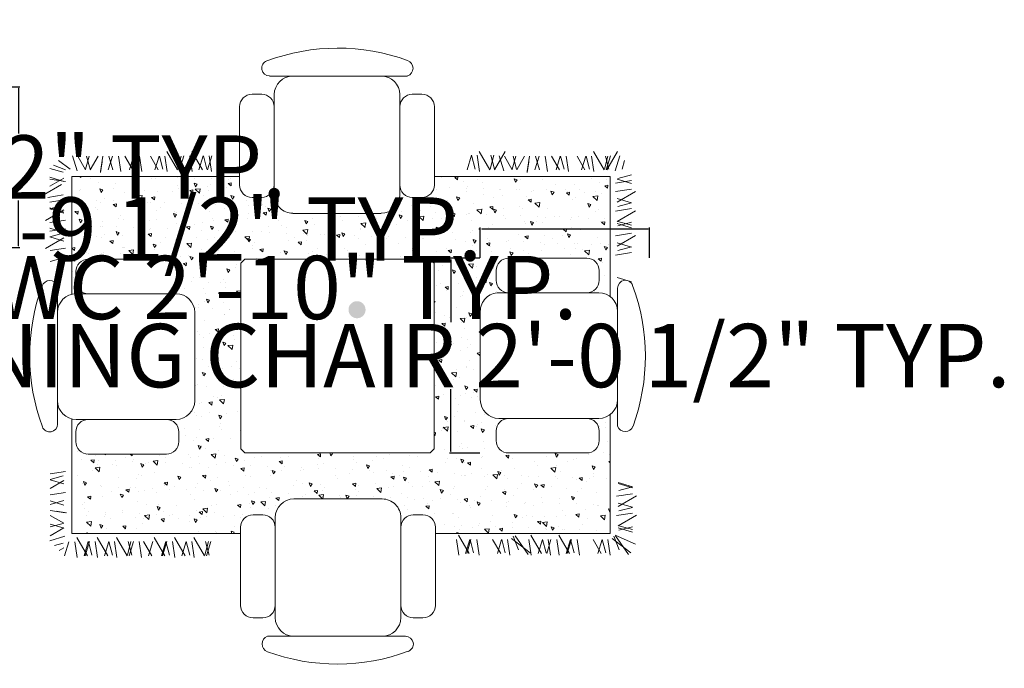
# Model space of a CAD drawing. Units: inches. Extents: x 638 to 1303, y 1 to 699.
# Tile 7 of 21: x 855 to 980, y 224 to 306. Entities that reach past the tile are written whole.
import ezdxf

# ---------------------------------------------------------------- set-up
doc = ezdxf.new("R2010")
doc.units = ezdxf.units.IN
doc.header["$MEASUREMENT"] = 0
for name, color, linetype, lineweight in [('A-ANNO-DIMS', 2, 'Continuous', 18), ('A-FURN-PATT', 8, 'Continuous', 13), ('A-FURN-RUGS', 8, 'Continuous', 13), ('Furniture', 7, 'Continuous', 15)]:
    doc.layers.add(name, color=color, linetype=linetype, lineweight=lineweight)
doc.styles.get("Standard").update_dxf_attribs({"font": 'arial.ttf'})
doc.dimstyles.get("Standard").update_dxf_attribs({"dimtxt": 8, "dimasz": 0.18, "dimexe": 0.18, "dimexo": 0.0625, "dimgap": 0.09, "dimtad": 0, "dimtih": 1, "dimtoh": 1, "dimdec": 4, "dimzin": 0, "dimdsep": 46, "dimlunit": 3, "dimtxsty": 'Standard', "dimcen": 0.09, "dimadec": 0, "dimazin": 0, "dimtfac": 1, "dimtdec": 4, "dimtofl": 0, "dimtmove": 0, "dimatfit": 3, "dimfxl": 1, "dimtolj": 1, "dimtzin": 0, "dimarcsym": 0})

# ---------------------------------------------------------------- blocks, each defined once
blk = doc.blocks.new('CHAIR-UPHOLSTERED')
for p, q in [((7.4, 24.61, 7.15), (17.29, 24.61, 7.15)), ((5.82, 21.82, 7.15), (5.82, 23.04, 7.15)), ((18.86, 23.04, 7.15), (18.86, 21.82, 7.15)), ((3.52, 21.23, 7.15), (3.52, 4.36, 7.15)), ((5.87, 20.25, 7.15), (18.51, 20.25, 7.15)), ((17.29, 20.25, 7.15), (7.4, 20.25, 7.15)), ((3.52, 6.72, 7.15), (3.52, 17.89, 7.15)), ((20.87, 17.89, 7.15), (20.87, 6.72, 7.15)), ((3.52, 4.36, 7.15), (3.52, 3.77, 7.15)), ((18.51, 4.36, 7.15), (5.87, 4.36, 7.15)), ((7.4, 4.36, 7.15), (17.29, 4.36, 7.15)), ((5.82, 1.57, 7.15), (5.82, 2.79, 7.15)), ((18.86, 2.79, 7.15), (18.86, 1.57, 7.15)), ((17.29, 0, 7.15), (7.4, 0, 7.15))]:
    blk.add_line(p, q)
for centre, radius, start, end in [((7.4, 23.04, 7.15), 1.57, 90, 180), ((17.29, 23.04, 7.15), 1.57, 0, 90), ((25.77, 12.4, 7.15), 25.77, 159.9544, 200.3611), ((2.54, 20.87, 7.15), 1.04, 20.0456, 159.9544), ((7.4, 21.82, 7.15), 1.57, 180, 270), ((17.29, 21.82, 7.15), 1.57, 270, 0), ((5.87, 17.89, 7.15), 2.35, 90, 180), ((18.51, 17.89, 7.15), 2.35, 0, 90), ((5.87, 6.72, 7.15), 2.35, 180, 270), ((18.51, 6.72, 7.15), 2.35, 270, 0), ((2.53, 3.77, 7.15), 0.986, 200.3611, 0), ((7.4, 2.79, 7.15), 1.57, 90, 180), ((17.29, 2.79, 7.15), 1.57, 0, 90), ((7.4, 1.57, 7.15), 1.57, 180, 270), ((17.29, 1.57, 7.15), 1.57, 270, 0)]:
    blk.add_arc(centre, radius, start, end)
blk = doc.blocks.new('*D30')
at = {"layer": 'A-ANNO-DIMS', "color": 0, "lineweight": -2, "transparency": 16777216}
for p, q in [((913.6, 276.19), (909.79, 276.19)), ((909.97, 276.01), (909.97, 268.11)), ((909.97, 251.76), (909.97, 259.66)), ((913.6, 251.58), (909.79, 251.58))]:
    blk.add_line(p, q, dxfattribs=at)
at = {"layer": 'A-ANNO-DIMS', "color": 0, "transparency": 16777216}
for points in [[(909.94, 276.01), (910, 276.01), (909.97, 276.19)], [(909.94, 251.76), (910, 251.76), (909.97, 251.58)]]:
    blk.add_solid(points, dxfattribs=at)
at = {"layer": 'Defpoints', "color": 0, "transparency": 16777216}
for p in [(913.67, 276.19), (909.97, 251.58), (913.67, 251.58)]:
    blk.add_point(p, dxfattribs=at)
at = {"layer": 'A-ANNO-DIMS', "color": 0, "transparency": 16777216, "insert": (909.97, 263.89), "char_height": 8, "attachment_point": 5}
blk.add_mtext('\\A1;DINING CHAIR 2\'-0 1/2" TYP.', dxfattribs=at)
blk = doc.blocks.new('*D31')
at = {"layer": 'A-ANNO-DIMS', "color": 0, "lineweight": -2, "transparency": 16777216}
for p, q in [((913.67, 276.25), (913.67, 280.06)), ((935.07, 276.25), (935.07, 280.06)), ((913.67, 279.88), (913.49, 279.88)), ((934.89, 279.88), (913.85, 279.88))]:
    blk.add_line(p, q, dxfattribs=at)
at = {"layer": 'A-ANNO-DIMS', "color": 0, "transparency": 16777216}
for points in [[(913.85, 279.91), (913.85, 279.85), (913.67, 279.88)], [(934.89, 279.91), (934.89, 279.85), (935.07, 279.88)]]:
    blk.add_solid(points, dxfattribs=at)
at = {"layer": 'Defpoints', "color": 0, "transparency": 16777216}
for p in [(913.67, 279.88), (913.67, 276.19), (935.07, 276.19)]:
    blk.add_point(p, dxfattribs=at)
at = {"layer": 'A-ANNO-DIMS', "color": 0, "transparency": 16777216, "insert": (880.07, 279.88), "char_height": 8, "attachment_point": 5}
blk.add_mtext('\\A1;1\'-9 1/2" TYP.', dxfattribs=at)
blk = doc.blocks.new('*D32')
at = {"layer": 'A-ANNO-DIMS', "color": 0, "lineweight": -2, "transparency": 16777216}
for p, q in [((816.4, 277.5), (816.4, 272.31)), ((850.23, 277.5), (850.23, 272.31)), ((816.58, 272.49), (850.05, 272.49)), ((850.23, 272.49), (850.41, 272.49))]:
    blk.add_line(p, q, dxfattribs=at)
at = {"layer": 'A-ANNO-DIMS', "color": 0, "transparency": 16777216}
for points in [[(816.58, 272.52), (816.58, 272.46), (816.4, 272.49)], [(850.05, 272.52), (850.05, 272.46), (850.23, 272.49)]]:
    blk.add_solid(points, dxfattribs=at)
at = {"layer": 'Defpoints', "color": 0, "transparency": 16777216}
for p in [(816.4, 277.56), (850.23, 277.56), (850.23, 272.49)]:
    blk.add_point(p, dxfattribs=at)
at = {"layer": 'A-ANNO-DIMS', "color": 0, "transparency": 16777216, "insert": (889.02, 272.49), "char_height": 8, "attachment_point": 5}
blk.add_mtext('\\A1;WC 2\'-10" TYP.', dxfattribs=at)
blk = doc.blocks.new('*D33')
at = {"layer": 'A-ANNO-DIMS', "color": 0, "lineweight": -2, "transparency": 16777216}
for p, q in [((850.3, 297.86), (855.49, 297.86)), ((855.31, 297.68), (855.31, 291.94)), ((855.31, 277.74), (855.31, 283.49)), ((850.3, 277.56), (855.49, 277.56))]:
    blk.add_line(p, q, dxfattribs=at)
at = {"layer": 'A-ANNO-DIMS', "color": 0, "transparency": 16777216}
for points in [[(855.28, 297.68), (855.34, 297.68), (855.31, 297.86)], [(855.28, 277.74), (855.34, 277.74), (855.31, 277.56)]]:
    blk.add_solid(points, dxfattribs=at)
at = {"layer": 'Defpoints', "color": 0, "transparency": 16777216}
for p in [(850.23, 297.86), (855.31, 297.86), (850.23, 277.56)]:
    blk.add_point(p, dxfattribs=at)
at = {"layer": 'A-ANNO-DIMS', "color": 0, "transparency": 16777216, "insert": (855.31, 287.71), "char_height": 8, "attachment_point": 5}
blk.add_mtext('\\A1;1\'-8 1/2" TYP.', dxfattribs=at)

msp = doc.modelspace()

# ---------------------------------------------------------------- hatches: boundary and pattern name
at = {"layer": 'A-FURN-PATT'}
h = msp.add_hatch(dxfattribs=at)
h.set_pattern_fill('AR-CONC', color=256, scale=0.643499, angle=90, style=0)
h.set_pattern_definition([(140, (0, 0), (0.403809, 4.61556), [0.482624, -5.308864]), (85, (0, 0), (-4.840347, -0.892863), [0.3861, -4.247092]), (190.45144, (0.0337, 0.3846), (-4.436537, 3.722697), [0.410167, -4.51184]), (136.1842, (-1.287, 1e-16), (1.065114, 6.867684), [0.723936, -7.963297]), (186.6356, (-1.198, 0.572), (-6.26844, 6.014538), [0.61525, -6.767765]), (81.1842, (-1.287, 1e-16), (-6.26844, 6.01454), [0.57915, -6.370637]), (111, (-0.9652, 0.6435), (2.590847, 3.841089), [0.482624, -5.308864]), (56, (-0.9652, 0.6435), (-4.666331, 1.56573), [0.3861, -4.247092]), (161.45144, (-0.7493, 0.9636), (-2.075484, 5.40682), [0.410167, -4.51184]), (127.5, (0, 0), (-2.1421677, 0.0782485), [0, -4.1956116, 0, -4.3114414, 0, -4.263179]), (97.5, (0, 0), (-2.5380343, 1.692849), [0, -2.458165, 0, -4.099087, 0, -1.624834]), (57.5, (-1e-16, -1.435), (0.1451403, 3.4351405), [0, -1.608747, 0, -5.01929, 0, -6.660212]), (47.5, (-1e-16, -2.0785), (-0.644174, 3.7527955), [0, -2.091371, 0, -3.333323, 0, -4.729716])])
h.paths.add_polyline_path([(883.26022, 286.50863), (862.04846, 286.50863), (862.04846, 271.63405), (862.11053, 271.64895), (862.23163, 271.67139), (862.35374, 271.68747), (862.47652, 271.69713), (862.59965, 271.70036), (864.1212, 271.70036), (864.03898, 271.70251), (863.95698, 271.70896), (863.87543, 271.7197), (863.79456, 271.73469), (863.71458, 271.75389), (863.63572, 271.77725), (863.55818, 271.80471), (863.48219, 271.83618), (863.40795, 271.87159), (863.33567, 271.91084), (863.26554, 271.95382), (863.19775, 272.00041), (863.1325, 272.05048), (863.06995, 272.10389), (863.01029, 272.16051), (862.95367, 272.22018), (862.90025, 272.28272), (862.85018, 272.34798), (862.80359, 272.41576), (862.76062, 272.48589), (862.72137, 272.55818), (862.68596, 272.63241), (862.65448, 272.70841), (862.62703, 272.78594), (862.60367, 272.8648), (862.58447, 272.94478), (862.56948, 273.02566), (862.55874, 273.1072), (862.55229, 273.1892), (862.55013, 273.27143), (862.55013, 274.49251), (862.55229, 274.57473), (862.55874, 274.65673), (862.56948, 274.73828), (862.58447, 274.81915), (862.60367, 274.89913), (862.62703, 274.978), (862.65448, 275.05553), (862.68596, 275.13152), (862.72137, 275.20576), (862.76062, 275.27804), (862.80359, 275.34817), (862.85018, 275.41596), (862.90025, 275.48121), (862.95367, 275.54376), (863.01029, 275.60342), (863.06995, 275.66004), (863.1325, 275.71346), (863.19775, 275.76353), (863.26554, 275.81012), (863.33567, 275.85309), (863.40795, 275.89234), (863.48219, 275.92775), (863.55818, 275.95923), (863.63572, 275.98668), (863.71458, 276.01004), (863.79456, 276.02925), (863.87543, 276.04424), (863.95698, 276.05497), (864.03898, 276.06142), (864.1212, 276.06358), (874.01311, 276.06358), (874.09533, 276.06142), (874.17733, 276.05497), (874.25888, 276.04424), (874.33975, 276.02925), (874.41973, 276.01004), (874.4986, 275.98668), (874.57613, 275.95923), (874.65212, 275.92775), (874.72636, 275.89234), (874.79864, 275.85309), (874.86878, 275.81012), (874.93656, 275.76353), (875.00182, 275.71346), (875.06436, 275.66004), (875.12402, 275.60342), (875.18064, 275.54376), (875.23406, 275.48121), (875.28413, 275.41596), (875.33072, 275.34817), (875.3737, 275.27804), (875.41294, 275.20576), (875.44835, 275.13152), (875.47983, 275.05553), (875.50729, 274.978), (875.53065, 274.89913), (875.54985, 274.81915), (875.56484, 274.73828), (875.57557, 274.65673), (875.58203, 274.57473), (875.58418, 274.49251), (875.58418, 273.27143), (875.58203, 273.1892), (875.57557, 273.1072), (875.56484, 273.02566), (875.54985, 272.94478), (875.53065, 272.8648), (875.50729, 272.78594), (875.47983, 272.70841), (875.44835, 272.63241), (875.41294, 272.55818), (875.3737, 272.48589), (875.33072, 272.41576), (875.28413, 272.34798), (875.23406, 272.28272), (875.18064, 272.22018), (875.12402, 272.16051), (875.06436, 272.10389), (875.00182, 272.05048), (874.93656, 272.00041), (874.86878, 271.95382), (874.79864, 271.91084), (874.72636, 271.87159), (874.65212, 271.83618), (874.57613, 271.80471), (874.4986, 271.77725), (874.41973, 271.75389), (874.33975, 271.73469), (874.25888, 271.7197), (874.17733, 271.70896), (874.09533, 271.70251), (874.01311, 271.70036), (875.24067, 271.70036), (875.36379, 271.69713), (875.48657, 271.68747), (875.60868, 271.67139), (875.72978, 271.64895), (875.84954, 271.6202), (875.96763, 271.58522), (876.08373, 271.5441), (876.19752, 271.49697), (876.30869, 271.44395), (876.41693, 271.38518), (876.52194, 271.32083), (876.62344, 271.25107), (876.72115, 271.17609), (876.81481, 271.0961), (876.90415, 271.01132), (876.98893, 270.92198), (877.06892, 270.82833), (877.14389, 270.73061), (877.21365, 270.62911), (877.27801, 270.5241), (877.33678, 270.41586), (877.3898, 270.30469), (877.43693, 270.19091), (877.47804, 270.07481), (877.51303, 269.95672), (877.54178, 269.83696), (877.56422, 269.71585), (877.5803, 269.59374), (877.58996, 269.47096), (877.59319, 269.34784), (877.59319, 258.1688), (877.58996, 258.04567), (877.5803, 257.92289), (877.56422, 257.80078), (877.54178, 257.67968), (877.51303, 257.55992), (877.47804, 257.44183), (877.43693, 257.32573), (877.3898, 257.21194), (877.33678, 257.10077), (877.27801, 256.99254), (877.21365, 256.88752), (877.14389, 256.78602), (877.06892, 256.68831), (876.98893, 256.59465), (876.90415, 256.50531), (876.81481, 256.42053), (876.72115, 256.34054), (876.62344, 256.26557), (876.52194, 256.19581), (876.41693, 256.13145), (876.30869, 256.07269), (876.19752, 256.01966), (876.08373, 255.97253), (875.96763, 255.93142), (875.84954, 255.89644), (875.72978, 255.86768), (875.60868, 255.84524), (875.48657, 255.82916), (875.36379, 255.8195), (875.24067, 255.81628), (874.01311, 255.81628), (874.09533, 255.81412), (874.17733, 255.80767), (874.25888, 255.79693), (874.33975, 255.78194), (874.41973, 255.76274), (874.4986, 255.73938), (874.57613, 255.71193), (874.65212, 255.68045), (874.72636, 255.64504), (874.79864, 255.60579), (874.86878, 255.56282), (874.93656, 255.51623), (875.00182, 255.46616), (875.06436, 255.41274), (875.12402, 255.35612), (875.18064, 255.29646), (875.23406, 255.23391), (875.28413, 255.16866), (875.33072, 255.10087), (875.3737, 255.03074), (875.41294, 254.95846), (875.44835, 254.88422), (875.47983, 254.80823), (875.50729, 254.73069), (875.53065, 254.65183), (875.54985, 254.57185), (875.56484, 254.49098), (875.57557, 254.40943), (875.58203, 254.32743), (875.58418, 254.24521), (875.58418, 253.02412), (875.58203, 252.9419), (875.57557, 252.8599), (875.56484, 252.77836), (875.54985, 252.69748), (875.53065, 252.6175), (875.50729, 252.53864), (875.47983, 252.4611), (875.44835, 252.38511), (875.41294, 252.31087), (875.3737, 252.23859), (875.33072, 252.16846), (875.28413, 252.10067), (875.23406, 252.03542), (875.18064, 251.97287), (875.12402, 251.91321), (875.06436, 251.85659), (875.00182, 251.80318), (874.93656, 251.7531), (874.86878, 251.70652), (874.79864, 251.66354), (874.72636, 251.62429), (874.65212, 251.58888), (874.57613, 251.55741), (874.4986, 251.52995), (874.41973, 251.50659), (874.33975, 251.48739), (874.25888, 251.4724), (874.17733, 251.46166), (874.09533, 251.45521), (874.01311, 251.45306), (864.1212, 251.45306), (864.03898, 251.45521), (863.95698, 251.46166), (863.87543, 251.4724), (863.79456, 251.48739), (863.71458, 251.50659), (863.63572, 251.52995), (863.55818, 251.55741), (863.48219, 251.58888), (863.40795, 251.62429), (863.33567, 251.66354), (863.26554, 251.70652), (863.19775, 251.7531), (863.1325, 251.80318), (863.06995, 251.85659), (863.01029, 251.91321), (862.95367, 251.97287), (862.90025, 252.03542), (862.85018, 252.10067), (862.80359, 252.16846), (862.76062, 252.23859), (862.72137, 252.31087), (862.68596, 252.38511), (862.65448, 252.4611), (862.62703, 252.53864), (862.60367, 252.6175), (862.58447, 252.69748), (862.56948, 252.77836), (862.55874, 252.8599), (862.55229, 252.9419), (862.55013, 253.02412), (862.55013, 254.24521), (862.55229, 254.32743), (862.55874, 254.40943), (862.56948, 254.49098), (862.58447, 254.57185), (862.60367, 254.65183), (862.62703, 254.73069), (862.65448, 254.80823), (862.68596, 254.88422), (862.72137, 254.95846), (862.76062, 255.03074), (862.80359, 255.10087), (862.85018, 255.16866), (862.90025, 255.23391), (862.95367, 255.29646), (863.01029, 255.35612), (863.06995, 255.41274), (863.1325, 255.46616), (863.19775, 255.51623), (863.26554, 255.56282), (863.33567, 255.60579), (863.40795, 255.64504), (863.48219, 255.68045), (863.55818, 255.71193), (863.63572, 255.73938), (863.71458, 255.76274), (863.79456, 255.78194), (863.87543, 255.79693), (863.95698, 255.80767), (864.03898, 255.81412), (864.1212, 255.81628), (862.59965, 255.81628), (862.47652, 255.8195), (862.35374, 255.82916), (862.23163, 255.84524), (862.11053, 255.86768), (862.04846, 255.88259), (862.04846, 241.41532), (883.3886, 241.41532), (883.3886, 242.20595), (883.39075, 242.28817), (883.39721, 242.37017), (883.40794, 242.45172), (883.42293, 242.53259), (883.44213, 242.61257), (883.4655, 242.69144), (883.49295, 242.76897), (883.52443, 242.84496), (883.55984, 242.9192), (883.59909, 242.99149), (883.64206, 243.06162), (883.68865, 243.1294), (883.73872, 243.19466), (883.79214, 243.2572), (883.84876, 243.31686), (883.90842, 243.37348), (883.97096, 243.4269), (884.03622, 243.47697), (884.104, 243.52356), (884.17414, 243.56654), (884.24642, 243.60578), (884.32066, 243.64119), (884.39665, 243.67267), (884.47418, 243.70013), (884.55305, 243.72349), (884.63303, 243.74269), (884.7139, 243.75768), (884.79545, 243.76841), (884.87745, 243.77487), (884.95967, 243.77702), (886.18075, 243.77702), (886.26298, 243.77487), (886.34498, 243.76841), (886.42652, 243.75768), (886.5074, 243.74269), (886.58738, 243.72349), (886.66624, 243.70013), (886.74377, 243.67267), (886.81976, 243.64119), (886.894, 243.60578), (886.96629, 243.56654), (887.03642, 243.52356), (887.1042, 243.47697), (887.16946, 243.4269), (887.232, 243.37348), (887.29167, 243.31686), (887.34828, 243.2572), (887.4017, 243.19466), (887.45177, 243.1294), (887.49836, 243.06162), (887.54134, 242.99149), (887.58059, 242.9192), (887.616, 242.84496), (887.64747, 242.76897), (887.67493, 242.69144), (887.69829, 242.61257), (887.71749, 242.53259), (887.73248, 242.45172), (887.74322, 242.37017), (887.74967, 242.28817), (887.75182, 242.20595), (887.75182, 243.43351), (887.75505, 243.55663), (887.76471, 243.67941), (887.78079, 243.80152), (887.80323, 243.92262), (887.83198, 244.04238), (887.86696, 244.16048), (887.90808, 244.27657), (887.95521, 244.39036), (888.00823, 244.50153), (888.067, 244.60977), (888.13135, 244.71478), (888.20111, 244.81628), (888.27609, 244.914), (888.35608, 245.00765), (888.44086, 245.09699), (888.5302, 245.18177), (888.62385, 245.26176), (888.72156, 245.33674), (888.82307, 245.4065), (888.92808, 245.47085), (889.03632, 245.52962), (889.14749, 245.58264), (889.26127, 245.62977), (889.37737, 245.67089), (889.49546, 245.70587), (889.61522, 245.73462), (889.73633, 245.75706), (889.85844, 245.77314), (889.98122, 245.7828), (890.10434, 245.78603), (901.28338, 245.78603), (901.40651, 245.7828), (901.52929, 245.77314), (901.6514, 245.75706), (901.7725, 245.73462), (901.89226, 245.70587), (902.01035, 245.67089), (902.12645, 245.62977), (902.24024, 245.58264), (902.35141, 245.52962), (902.45964, 245.47085), (902.56466, 245.4065), (902.66616, 245.33674), (902.76387, 245.26176), (902.85753, 245.18177), (902.94687, 245.09699), (903.03165, 245.00765), (903.11163, 244.914), (903.18661, 244.81628), (903.25637, 244.71478), (903.32073, 244.60977), (903.37949, 244.50153), (903.43252, 244.39036), (903.47965, 244.27657), (903.52076, 244.16048), (903.55574, 244.04238), (903.5845, 243.92262), (903.60694, 243.80152), (903.62302, 243.67941), (903.63268, 243.55663), (903.6359, 243.43351), (903.6359, 242.20595), (903.63806, 242.28817), (903.64451, 242.37017), (903.65525, 242.45172), (903.67023, 242.53259), (903.68944, 242.61257), (903.7128, 242.69144), (903.74025, 242.76897), (903.77173, 242.84496), (903.80714, 242.9192), (903.84639, 242.99149), (903.88936, 243.06162), (903.93595, 243.1294), (903.98602, 243.19466), (904.03944, 243.2572), (904.09606, 243.31686), (904.15572, 243.37348), (904.21827, 243.4269), (904.28352, 243.47697), (904.35131, 243.52356), (904.42144, 243.56654), (904.49372, 243.60578), (904.56796, 243.64119), (904.64395, 243.67267), (904.72148, 243.70013), (904.80035, 243.72349), (904.88033, 243.74269), (904.9612, 243.75768), (905.04275, 243.76841), (905.12475, 243.77487), (905.20697, 243.77702), (906.42806, 243.77702), (906.51028, 243.77487), (906.59228, 243.76841), (906.67382, 243.75768), (906.7547, 243.74269), (906.83468, 243.72349), (906.91354, 243.70013), (906.99108, 243.67267), (907.06707, 243.64119), (907.14131, 243.60578), (907.21359, 243.56654), (907.28372, 243.52356), (907.35151, 243.47697), (907.41676, 243.4269), (907.4793, 243.37348), (907.53897, 243.31686), (907.59559, 243.2572), (907.649, 243.19466), (907.69908, 243.1294), (907.74566, 243.06162), (907.78864, 242.99149), (907.82789, 242.9192), (907.8633, 242.84496), (907.89477, 242.76897), (907.92223, 242.69144), (907.94559, 242.61257), (907.96479, 242.53259), (907.97978, 242.45172), (907.99052, 242.37017), (907.99697, 242.28817), (907.99912, 242.20595), (907.99912, 241.41532), (930.08632, 241.41532), (930.08632, 256.4276), (930.04247, 256.39395), (929.94097, 256.32419), (929.83595, 256.25984), (929.72771, 256.20107), (929.61655, 256.14805), (929.50276, 256.10092), (929.38666, 256.0598), (929.26857, 256.02482), (929.14881, 255.99607), (929.02771, 255.97363), (928.9056, 255.95755), (928.78281, 255.94789), (928.65969, 255.94466), (927.13814, 255.94466), (927.22036, 255.94251), (927.30236, 255.93606), (927.38391, 255.92532), (927.46478, 255.91033), (927.54476, 255.89113), (927.62362, 255.86777), (927.70116, 255.84031), (927.77715, 255.80884), (927.85139, 255.77343), (927.92367, 255.73418), (927.9938, 255.6912), (928.06159, 255.64462), (928.12684, 255.59454), (928.18939, 255.54113), (928.24905, 255.48451), (928.30567, 255.42484), (928.35909, 255.3623), (928.40916, 255.29705), (928.45575, 255.22926), (928.49872, 255.15913), (928.53797, 255.08684), (928.57338, 255.01261), (928.60485, 254.93662), (928.63231, 254.85908), (928.65567, 254.78022), (928.67487, 254.70024), (928.68986, 254.61936), (928.7006, 254.53782), (928.70705, 254.45582), (928.7092, 254.37359), (928.7092, 253.15251), (928.70705, 253.07029), (928.7006, 252.98829), (928.68986, 252.90674), (928.67487, 252.82587), (928.65567, 252.74589), (928.63231, 252.66702), (928.60485, 252.58949), (928.57338, 252.5135), (928.53797, 252.43926), (928.49872, 252.36698), (928.45575, 252.29685), (928.40916, 252.22906), (928.35909, 252.16381), (928.30567, 252.10126), (928.24905, 252.0416), (928.18939, 251.98498), (928.12684, 251.93156), (928.06159, 251.88149), (927.9938, 251.8349), (927.92367, 251.79193), (927.85139, 251.75268), (927.77715, 251.71727), (927.70116, 251.68579), (927.62362, 251.65834), (927.54476, 251.63498), (927.46478, 251.61577), (927.38391, 251.60079), (927.30236, 251.59005), (927.22036, 251.5836), (927.13814, 251.58144), (917.24623, 251.58144), (917.164, 251.5836), (917.08201, 251.59005), (917.00046, 251.60079), (916.91958, 251.61577), (916.83961, 251.63498), (916.76074, 251.65834), (916.68321, 251.68579), (916.60722, 251.71727), (916.53298, 251.75268), (916.46069, 251.79193), (916.39056, 251.8349), (916.32278, 251.88149), (916.25752, 251.93156), (916.19498, 251.98498), (916.13532, 252.0416), (916.0787, 252.10126), (916.02528, 252.16381), (915.97521, 252.22906), (915.92862, 252.29685), (915.88564, 252.36698), (915.8464, 252.43926), (915.81099, 252.5135), (915.77951, 252.58949), (915.75205, 252.66702), (915.72869, 252.74589), (915.70949, 252.82587), (915.6945, 252.90674), (915.68377, 252.98829), (915.67731, 253.07029), (915.67516, 253.15251), (915.67516, 254.37359), (915.67731, 254.45582), (915.68377, 254.53782), (915.6945, 254.61936), (915.70949, 254.70024), (915.72869, 254.78022), (915.75205, 254.85908), (915.77951, 254.93662), (915.81099, 255.01261), (915.8464, 255.08684), (915.88564, 255.15913), (915.92862, 255.22926), (915.97521, 255.29705), (916.02528, 255.3623), (916.0787, 255.42484), (916.13532, 255.48451), (916.19498, 255.54113), (916.25752, 255.59454), (916.32278, 255.64462), (916.39056, 255.6912), (916.46069, 255.73418), (916.53298, 255.77343), (916.60722, 255.80884), (916.68321, 255.84031), (916.76074, 255.86777), (916.83961, 255.89113), (916.91958, 255.91033), (917.00046, 255.92532), (917.08201, 255.93606), (917.164, 255.94251), (917.24623, 255.94466), (916.01867, 255.94466), (915.89555, 255.94789), (915.77277, 255.95755), (915.65066, 255.97363), (915.52956, 255.99607), (915.4098, 256.02482), (915.2917, 256.0598), (915.1756, 256.10092), (915.06182, 256.14805), (914.95065, 256.20107), (914.84241, 256.25984), (914.7374, 256.32419), (914.6359, 256.39395), (914.53818, 256.46893), (914.44453, 256.54892), (914.35519, 256.6337), (914.27041, 256.72304), (914.19042, 256.81669), (914.11544, 256.91441), (914.04568, 257.01591), (913.98133, 257.12092), (913.92256, 257.22916), (913.86954, 257.34033), (913.82241, 257.45411), (913.78129, 257.57021), (913.74631, 257.6883), (913.71756, 257.80807), (913.69512, 257.92917), (913.67904, 258.05128), (913.66938, 258.17406), (913.66615, 258.29718), (913.66615, 269.47623), (913.66938, 269.59935), (913.67904, 269.72213), (913.69512, 269.84424), (913.71756, 269.96534), (913.74631, 270.0851), (913.78129, 270.20319), (913.82241, 270.31929), (913.86954, 270.43308), (913.92256, 270.54425), (913.98133, 270.65248), (914.04568, 270.7575), (914.11544, 270.859), (914.19042, 270.95671), (914.27041, 271.05037), (914.35519, 271.13971), (914.44453, 271.22449), (914.53818, 271.30448), (914.6359, 271.37945), (914.7374, 271.44921), (914.84241, 271.51357), (914.95065, 271.57234), (915.06182, 271.62536), (915.1756, 271.67249), (915.2917, 271.7136), (915.4098, 271.74858), (915.52956, 271.77734), (915.65066, 271.79978), (915.77277, 271.81586), (915.89555, 271.82552), (916.01867, 271.82874), (917.24623, 271.82874), (917.164, 271.8309), (917.08201, 271.83735), (917.00046, 271.84809), (916.91958, 271.86308), (916.83961, 271.88228), (916.76074, 271.90564), (916.68321, 271.93309), (916.60722, 271.96457), (916.53298, 271.99998), (916.46069, 272.03923), (916.39056, 272.0822), (916.32278, 272.12879), (916.25752, 272.17886), (916.19498, 272.23228), (916.13532, 272.2889), (916.0787, 272.34856), (916.02528, 272.41111), (915.97521, 272.47636), (915.92862, 272.54415), (915.88564, 272.61428), (915.8464, 272.68656), (915.81099, 272.7608), (915.77951, 272.83679), (915.75205, 272.91433), (915.72869, 272.99319), (915.70949, 273.07317), (915.6945, 273.15404), (915.68377, 273.23559), (915.67731, 273.31759), (915.67516, 273.39981), (915.67516, 274.6209), (915.67731, 274.70312), (915.68377, 274.78512), (915.6945, 274.86667), (915.70949, 274.94754), (915.72869, 275.02752), (915.75205, 275.10638), (915.77951, 275.18392), (915.81099, 275.25991), (915.8464, 275.33415), (915.88564, 275.40643), (915.92862, 275.47656), (915.97521, 275.54435), (916.02528, 275.6096), (916.0787, 275.67215), (916.13532, 275.73181), (916.19498, 275.78843), (916.25752, 275.84185), (916.32278, 275.89192), (916.39056, 275.9385), (916.46069, 275.98148), (916.53298, 276.02073), (916.60722, 276.05614), (916.68321, 276.08761), (916.76074, 276.11507), (916.83961, 276.13843), (916.91958, 276.15763), (917.00046, 276.17262), (917.08201, 276.18336), (917.164, 276.18981), (917.24623, 276.19196), (927.13814, 276.19196), (927.22036, 276.18981), (927.30236, 276.18336), (927.38391, 276.17262), (927.46478, 276.15763), (927.54476, 276.13843), (927.62362, 276.11507), (927.70116, 276.08761), (927.77715, 276.05614), (927.85139, 276.02073), (927.92367, 275.98148), (927.9938, 275.9385), (928.06159, 275.89192), (928.12684, 275.84185), (928.18939, 275.78843), (928.24905, 275.73181), (928.30567, 275.67215), (928.35909, 275.6096), (928.40916, 275.54435), (928.45575, 275.47656), (928.49872, 275.40643), (928.53797, 275.33415), (928.57338, 275.25991), (928.60485, 275.18392), (928.63231, 275.10638), (928.65567, 275.02752), (928.67487, 274.94754), (928.68986, 274.86667), (928.7006, 274.78512), (928.70705, 274.70312), (928.7092, 274.6209), (928.7092, 273.39981), (928.70705, 273.31759), (928.7006, 273.23559), (928.68986, 273.15404), (928.67487, 273.07317), (928.65567, 272.99319), (928.63231, 272.91433), (928.60485, 272.83679), (928.57338, 272.7608), (928.53797, 272.68656), (928.49872, 272.61428), (928.45575, 272.54415), (928.40916, 272.47636), (928.35909, 272.41111), (928.30567, 272.34856), (928.24905, 272.2889), (928.18939, 272.23228), (928.12684, 272.17886), (928.06159, 272.12879), (927.9938, 272.0822), (927.92367, 272.03923), (927.85139, 271.99998), (927.77715, 271.96457), (927.70116, 271.93309), (927.62362, 271.90564), (927.54476, 271.88228), (927.46478, 271.86308), (927.38391, 271.84809), (927.30236, 271.83735), (927.22036, 271.8309), (927.13814, 271.82874), (928.65969, 271.82874), (928.78281, 271.82552), (928.9056, 271.81586), (929.02771, 271.79978), (929.14881, 271.77734), (929.26857, 271.74858), (929.38666, 271.7136), (929.50276, 271.67249), (929.61655, 271.62536), (929.72771, 271.57234), (929.83595, 271.51357), (929.94097, 271.44921), (930.04247, 271.37945), (930.08632, 271.3458), (930.08632, 286.50863), (907.87074, 286.50863), (907.87074, 285.43907), (907.86858, 285.35685), (907.86213, 285.27485), (907.85139, 285.1933), (907.83641, 285.11243), (907.8172, 285.03245), (907.79384, 284.95358), (907.76639, 284.87605), (907.73491, 284.80006), (907.6995, 284.72582), (907.66025, 284.65353), (907.61728, 284.5834), (907.57069, 284.51562), (907.52062, 284.45036), (907.4672, 284.38782), (907.41058, 284.32816), (907.35092, 284.27154), (907.28837, 284.21812), (907.22312, 284.16805), (907.15533, 284.12146), (907.0852, 284.07848), (907.01292, 284.03924), (906.93868, 284.00383), (906.86269, 283.97235), (906.78516, 283.94489), (906.70629, 283.92153), (906.62631, 283.90233), (906.54544, 283.88734), (906.46389, 283.87661), (906.38189, 283.87015), (906.29967, 283.868), (905.07858, 283.868), (904.99636, 283.87015), (904.91436, 283.87661), (904.83282, 283.88734), (904.75194, 283.90233), (904.67196, 283.92153), (904.5931, 283.94489), (904.51556, 283.97235), (904.43957, 284.00383), (904.36533, 284.03924), (904.29305, 284.07848), (904.22292, 284.12146), (904.15513, 284.16805), (904.08988, 284.21812), (904.02734, 284.27154), (903.96767, 284.32816), (903.91105, 284.38782), (903.85764, 284.45036), (903.80756, 284.51562), (903.76098, 284.5834), (903.718, 284.65353), (903.67875, 284.72582), (903.64334, 284.80006), (903.61187, 284.87605), (903.58441, 284.95358), (903.56105, 285.03245), (903.54185, 285.11243), (903.52686, 285.1933), (903.51612, 285.27485), (903.50967, 285.35685), (903.50752, 285.43907), (903.50752, 284.21151), (903.50429, 284.08839), (903.49463, 283.96561), (903.47855, 283.8435), (903.45611, 283.7224), (903.42736, 283.60264), (903.39238, 283.48454), (903.35126, 283.36845), (903.30413, 283.25466), (903.25111, 283.14349), (903.19234, 283.03525), (903.12799, 282.93024), (903.05823, 282.82874), (902.98325, 282.73102), (902.90326, 282.63737), (902.81848, 282.54803), (902.72914, 282.46325), (902.63549, 282.38326), (902.53777, 282.30829), (902.43627, 282.23852), (902.33126, 282.17417), (902.22302, 282.1154), (902.11185, 282.06238), (901.99807, 282.01525), (901.88197, 281.97413), (901.76387, 281.93915), (901.64411, 281.9104), (901.52301, 281.88796), (901.4009, 281.87188), (901.27812, 281.86222), (901.155, 281.85899), (889.97595, 281.85899), (889.85283, 281.86222), (889.73005, 281.87188), (889.60794, 281.88796), (889.48684, 281.9104), (889.36708, 281.93915), (889.24899, 281.97413), (889.13289, 282.01525), (889.0191, 282.06238), (888.90793, 282.1154), (888.79969, 282.17417), (888.69468, 282.23852), (888.59318, 282.30829), (888.49547, 282.38326), (888.40181, 282.46325), (888.31247, 282.54803), (888.22769, 282.63737), (888.1477, 282.73102), (888.07273, 282.82874), (888.00297, 282.93024), (887.93861, 283.03525), (887.87984, 283.14349), (887.82682, 283.25466), (887.77969, 283.36845), (887.73858, 283.48454), (887.7036, 283.60264), (887.67484, 283.7224), (887.6524, 283.8435), (887.63632, 283.96561), (887.62666, 284.08839), (887.62344, 284.21151), (887.62344, 285.43907), (887.62128, 285.35685), (887.61483, 285.27485), (887.60409, 285.1933), (887.5891, 285.11243), (887.5699, 285.03245), (887.54654, 284.95358), (887.51909, 284.87605), (887.48761, 284.80006), (887.4522, 284.72582), (887.41295, 284.65353), (887.36998, 284.5834), (887.32339, 284.51562), (887.27332, 284.45036), (887.2199, 284.38782), (887.16328, 284.32816), (887.10362, 284.27154), (887.04107, 284.21812), (886.97582, 284.16805), (886.90803, 284.12146), (886.8379, 284.07848), (886.76562, 284.03924), (886.69138, 284.00383), (886.61539, 283.97235), (886.53785, 283.94489), (886.45899, 283.92153), (886.37901, 283.90233), (886.29814, 283.88734), (886.21659, 283.87661), (886.13459, 283.87015), (886.05237, 283.868), (884.83128, 283.868), (884.74906, 283.87015), (884.66706, 283.87661), (884.58551, 283.88734), (884.50464, 283.90233), (884.42466, 283.92153), (884.3458, 283.94489), (884.26826, 283.97235), (884.19227, 284.00383), (884.11803, 284.03924), (884.04575, 284.07848), (883.97562, 284.12146), (883.90783, 284.16805), (883.84258, 284.21812), (883.78003, 284.27154), (883.72037, 284.32816), (883.66375, 284.38782), (883.61033, 284.45036), (883.56026, 284.51562), (883.51367, 284.5834), (883.4707, 284.65353), (883.43145, 284.72582), (883.39604, 284.80006), (883.36457, 284.87605), (883.33711, 284.95358), (883.31375, 285.03245), (883.29455, 285.11243), (883.27956, 285.1933), (883.26882, 285.27485), (883.26237, 285.35685), (883.26022, 285.43907)])
h.paths.add_polyline_path([(907.86314, 275.54625), (907.86314, 252.09877), (907.35341, 251.58904), (883.90593, 251.58904), (883.3962, 252.09877), (883.3962, 275.54625), (883.90593, 276.05598), (907.35341, 276.05598)], flags=0)
msp.add_hatch(color=256, dxfattribs=at).paths.add_polyline_path([(899.17645, 269.68268, 1), (897.01649, 269.68268, 1)])

# ---------------------------------------------------------------- linework, layer by layer
at = {"layer": 'A-FURN-RUGS'}
for p, q in [((862.13427, 289.13674, 7.14696), (862.71325, 287.21858, 7.14696)), ((862.79139, 289.06722, 7.14696), (863.7822, 287.36244, 7.14696)), ((864.22773, 289.07106, 7.14696), (863.79856, 287.43873, 7.14696)), ((863.92013, 289.07024, 7.14696), (864.34909, 287.43873, 7.14696)), ((865.36024, 289.07408, 7.14696), (864.36544, 287.36244, 7.14696)), ((865.96646, 289.0757, 7.14696), (865.67539, 287.14748, 7.14696)), ((867.1782, 289.07893, 7.14696), (866.65895, 287.35864, 7.14696)), ((866.72559, 289.07773, 7.14696), (867.24447, 287.35864, 7.14696)), ((867.93617, 289.08096, 7.14696), (868.22803, 287.14748, 7.14696)), ((868.76824, 289.08318, 7.14696), (869.76833, 287.36244, 7.14696)), ((869.85647, 289.08608, 7.14696), (869.33506, 287.35864, 7.14696)), ((869.90205, 289.08621, 7.14696), (870.33521, 287.43873, 7.14696)), ((870.61121, 289.0881, 7.14696), (870.90415, 287.14748, 7.14696)), ((871.97651, 289.09174, 7.14696), (872.98157, 287.36244, 7.14696)), ((873.0723, 289.09467, 7.14696), (872.5483, 287.35864, 7.14696)), ((873.11304, 289.09478, 7.14696), (873.54845, 287.43873, 7.14696)), ((873.82315, 289.09667, 7.14696), (874.11739, 287.14748, 7.14696)), ((874.07804, 289.68404, 7.14696), (875.42734, 287.36244, 7.14696)), ((875.88105, 289.10217, 7.14696), (875.44369, 287.43873, 7.14696)), ((875.55709, 289.1013, 7.14696), (875.99422, 287.43873, 7.14696)), ((876.19998, 289.10302, 7.14696), (875.67345, 287.35864, 7.14696)), ((876.94705, 289.10501, 7.14696), (877.24254, 287.14748, 7.14696)), ((877.20319, 289.68404, 7.14696), (878.55249, 287.36244, 7.14696)), ((878.64772, 289.10955, 7.14696), (878.11922, 287.35864, 7.14696)), ((878.68005, 289.10964, 7.14696), (879.11937, 287.43873, 7.14696)), ((879.7356, 289.11246, 7.14696), (879.20623, 287.35864, 7.14696)), ((879.39183, 289.11154, 7.14696), (879.68831, 287.14748, 7.14696)), ((912.57412, 289.20012, 7.14696), (912.01829, 287.35864, 7.14696)), ((912.55534, 289.20007, 7.14696), (913.01844, 287.43873, 7.14696)), ((913.27724, 289.202, 7.14696), (913.58737, 287.14748, 7.14696)), ((913.54802, 289.68404, 7.14696), (914.89732, 287.36244, 7.14696)), ((915.37876, 289.20761, 7.14696), (914.91368, 287.43873, 7.14696)), ((914.9994, 289.2066, 7.14696), (915.46421, 287.43873, 7.14696)), ((916.82986, 289.68404, 7.14696), (915.48056, 287.36244, 7.14696)), ((916.05407, 289.13674, 7.14696), (916.63304, 287.21858, 7.14696)), ((916.71118, 289.06722, 7.14696), (917.70199, 287.36244, 7.14696)), ((918.14752, 289.07106, 7.14696), (917.71835, 287.43873, 7.14696)), ((917.83992, 289.07024, 7.14696), (918.26888, 287.43873, 7.14696)), ((919.28003, 289.07408, 7.14696), (918.28523, 287.36244, 7.14696)), ((919.88625, 289.0757, 7.14696), (919.59518, 287.14748, 7.14696)), ((921.09799, 289.07893, 7.14696), (920.57874, 287.35864, 7.14696)), ((920.64538, 289.07773, 7.14696), (921.16427, 287.35864, 7.14696)), ((921.85596, 289.08096, 7.14696), (922.14782, 287.14748, 7.14696)), ((922.68803, 289.08318, 7.14696), (923.68812, 287.36244, 7.14696)), ((923.77626, 289.08608, 7.14696), (923.25485, 287.35864, 7.14696)), ((923.82184, 289.08621, 7.14696), (924.255, 287.43873, 7.14696)), ((924.531, 289.0881, 7.14696), (924.82394, 287.14748, 7.14696)), ((925.8963, 289.09174, 7.14696), (926.90136, 287.36244, 7.14696)), ((926.9921, 289.09467, 7.14696), (926.4681, 287.35864, 7.14696)), ((927.03283, 289.09478, 7.14696), (927.46825, 287.43873, 7.14696)), ((927.74295, 289.09667, 7.14696), (928.03718, 287.14748, 7.14696)), ((927.99783, 289.68404, 7.14696), (929.34713, 287.36244, 7.14696)), ((929.80084, 289.10217, 7.14696), (929.36348, 287.43873, 7.14696)), ((929.47689, 289.1013, 7.14696), (929.91401, 287.43873, 7.14696)), ((930.11977, 289.10302, 7.14696), (929.59325, 287.35864, 7.14696)), ((931.01249, 289.68404, 7.14696), (929.66319, 287.36244, 7.14696)), ((931.31112, 289.13674, 7.14696), (930.73214, 287.21858, 7.14696)), ((859.27165, 287.50898, 7.14696), (860.96267, 287.06437, 7.14696)), ((859.75367, 287.93526, 7.14696), (861.26571, 287.36244, 7.14696)), ((860.36277, 288.54436, 7.14696), (861.8326, 287.43873, 7.14696)), ((865.88702, 288.34917, 7.14696), (865.68448, 287.00741, 7.14696)), ((919.80681, 288.34917, 7.14696), (919.60427, 287.00741, 7.14696)), ((931.90349, 288.54436, 7.14696), (931.6128, 287.43873, 7.14696)), ((859.2717, 286.42212, 7.14696), (861.04276, 285.88755, 7.14696)), ((859.27471, 285.29544, 7.14696), (861.03896, 286.32082, 7.14696)), ((862.04846, 271.63488, 7.14696), (862.04846, 286.50863, 7.14696)), ((862.04846, 286.50863, 7.14696), (883.26022, 286.50863, 7.14696)), ((907.87074, 286.50863, 7.14696), (930.08632, 286.50863, 7.14696)), ((930.08632, 286.50863, 7.14696), (930.08632, 271.34681, 7.14696)), ((932.77252, 286.71029, 7.14696), (931.03547, 286.25358, 7.14696)), ((858.43516, 284.13642, 7.14696), (860.75676, 285.48572, 7.14696)), ((859.26974, 286.17367, 7.14696), (861.25392, 285.87416, 7.14696)), ((932.77444, 285.99111, 7.14696), (930.74421, 285.68464, 7.14696)), ((932.77544, 285.61735, 7.14696), (930.95538, 286.16672, 7.14696)), ((859.00476, 283.87886, 7.14696), (860.97173, 284.17577, 7.14696)), ((932.77734, 284.90454, 7.14696), (930.74421, 284.59763, 7.14696)), ((932.78197, 283.16961, 7.14696), (930.95538, 283.72095, 7.14696)), ((933.28077, 284.63699, 7.14696), (930.95917, 283.28769, 7.14696)), ((859.28007, 283.28821, 7.14696), (861.25392, 283.58617, 7.14696)), ((859.28204, 282.54854, 7.14696), (861.04276, 282.01708, 7.14696)), ((859.28234, 282.43956, 7.14696), (860.96267, 282.88136, 7.14696)), ((932.78194, 283.17999, 7.14696), (931.03547, 282.7208, 7.14696)), ((858.71736, 280.96518, 7.14696), (861.03896, 282.31448, 7.14696)), ((859.28241, 282.41255, 7.14696), (861.04276, 281.88121, 7.14696)), ((932.78387, 282.45976, 7.14696), (930.74421, 282.15187, 7.14696)), ((933.28077, 282.19122, 7.14696), (930.95917, 280.84192, 7.14696)), ((859.28696, 280.70761, 7.14696), (861.25392, 281.00453, 7.14696)), ((932.79032, 280.04194, 7.14696), (930.95538, 280.5958, 7.14696)), ((932.78946, 280.3644, 7.14696), (931.03547, 280.82556, 7.14696)), ((932.78847, 280.73594, 7.14696), (931.03547, 280.27503, 7.14696)), ((858.71736, 277.4324, 7.14696), (861.03896, 278.7817, 7.14696)), ((859.28894, 279.96481, 7.14696), (861.04276, 279.43544, 7.14696)), ((859.28986, 279.62104, 7.14696), (861.25392, 279.91752, 7.14696)), ((859.29176, 278.90926, 7.14696), (860.96267, 279.34858, 7.14696)), ((859.29185, 278.87693, 7.14696), (861.04276, 278.34843, 7.14696)), ((932.79221, 279.33586, 7.14696), (930.74421, 279.02672, 7.14696)), ((933.28077, 279.06607, 7.14696), (930.95917, 277.71677, 7.14696)), ((932.79686, 277.5942, 7.14696), (930.95538, 278.15003, 7.14696)), ((932.79681, 277.61298, 7.14696), (931.03547, 277.14988, 7.14696)), ((859.29639, 277.17626, 7.14696), (861.25392, 277.47175, 7.14696)), ((932.79873, 276.89108, 7.14696), (930.74421, 276.58095, 7.14696)), ((859.3001, 275.7863, 7.14696), (860.96267, 276.22343, 7.14696)), ((932.78197, 273.18491, 7.14696), (930.95538, 273.73625, 7.14696)), ((930.08632, 256.4266, 7.14696), (930.08632, 253.59857, 7.14696)), ((862.04846, 253.59857, 7.14696), (862.04846, 255.88176, 7.14696)), ((862.04846, 241.41532, 7.14696), (862.04846, 253.59857, 7.14696)), ((930.08632, 253.59857, 7.14696), (930.08632, 241.41532, 7.14696)), ((859.3133, 248.95734, 7.14696), (861.25392, 249.25028, 7.14696)), ((859.31519, 248.24819, 7.14696), (860.96267, 248.68135, 7.14696)), ((859.31532, 248.20261, 7.14696), (861.04276, 247.6812, 7.14696)), ((859.31822, 247.11438, 7.14696), (861.03896, 248.11446, 7.14696)), ((932.89953, 247.30238, 7.14696), (931.10416, 247.8443, 7.14696)), ((932.89989, 247.1664, 7.14696), (931.10416, 247.70843, 7.14696)), ((859.32044, 246.28231, 7.14696), (861.25392, 246.57417, 7.14696)), ((932.90183, 246.44258, 7.14696), (930.89299, 246.13934, 7.14696)), ((932.89955, 247.29514, 7.14696), (931.18425, 246.84415, 7.14696)), ((859.32247, 245.52434, 7.14696), (861.04276, 245.00508, 7.14696)), ((859.32367, 245.07173, 7.14696), (861.04276, 245.59061, 7.14696)), ((932.90643, 244.71866, 7.14696), (931.10416, 245.26266, 7.14696)), ((933.42955, 246.17869, 7.14696), (931.10795, 244.82939, 7.14696)), ((859.3257, 244.3126, 7.14696), (861.25392, 244.02153, 7.14696)), ((860.05223, 244.23316, 7.14696), (861.39399, 244.03062, 7.14696)), ((932.90835, 243.9978, 7.14696), (930.89299, 243.69357, 7.14696)), ((932.90644, 244.71531, 7.14696), (931.18425, 244.26251, 7.14696)), ((859.32732, 243.70638, 7.14696), (861.03896, 242.71158, 7.14696)), ((859.33116, 242.26626, 7.14696), (860.96267, 242.69522, 7.14696)), ((933.42955, 243.73292, 7.14696), (931.10795, 242.38362, 7.14696)), ((859.33034, 242.57387, 7.14696), (860.96267, 242.14469, 7.14696)), ((859.33418, 241.13753, 7.14696), (861.03896, 242.12834, 7.14696)), ((872.89526, 241.41532, 7.14696), (862.04846, 241.41532, 7.14696)), ((883.3886, 241.41532, 7.14696), (872.5623, 241.41532, 7.14696)), ((930.08632, 241.41532, 7.14696), (907.99912, 241.41532, 7.14696)), ((932.91478, 241.59099, 7.14696), (931.10416, 242.13751, 7.14696)), ((932.91392, 241.9125, 7.14696), (931.18425, 242.36727, 7.14696)), ((932.91296, 242.27126, 7.14696), (931.18425, 241.81674, 7.14696)), ((859.26466, 240.48041, 7.14696), (861.18282, 241.05939, 7.14696)), ((859.85703, 239.88804, 7.14696), (860.96267, 240.17873, 7.14696)), ((861.68556, 240.37786, 7.14696), (861.14561, 238.58902, 7.14696)), ((862.4125, 240.3798, 7.14696), (862.7147, 238.37785, 7.14696)), ((862.67535, 240.91441, 7.14696), (864.02465, 238.59281, 7.14696)), ((864.1333, 240.38439, 7.14696), (863.59138, 238.58902, 7.14696)), ((864.26928, 240.38475, 7.14696), (863.72725, 238.58902, 7.14696)), ((864.14054, 240.38441, 7.14696), (864.59153, 238.6691, 7.14696)), ((864.9931, 240.38669, 7.14696), (865.29634, 238.37785, 7.14696)), ((865.25699, 240.91441, 7.14696), (866.60629, 238.59281, 7.14696)), ((866.71702, 240.39129, 7.14696), (866.17302, 238.58902, 7.14696)), ((866.72037, 240.3913, 7.14696), (867.17317, 238.6691, 7.14696)), ((867.43788, 240.39321, 7.14696), (867.74211, 238.37785, 7.14696)), ((867.70276, 240.91441, 7.14696), (869.05206, 238.59281, 7.14696)), ((869.52318, 240.39878, 7.14696), (869.06841, 238.6691, 7.14696)), ((869.16442, 240.39782, 7.14696), (869.61894, 238.6691, 7.14696)), ((869.84469, 240.39964, 7.14696), (869.29817, 238.58902, 7.14696)), ((870.56178, 240.40155, 7.14696), (870.86726, 238.37785, 7.14696)), ((871.1251, 240.40306, 7.14696), (872.17721, 238.59281, 7.14696)), ((872.29243, 240.40617, 7.14696), (871.74394, 238.58902, 7.14696)), ((872.46189, 240.91441, 7.14696), (873.81119, 238.59281, 7.14696)), ((873.91984, 240.38439, 7.14696), (873.37793, 238.58902, 7.14696)), ((874.05583, 240.38475, 7.14696), (873.5138, 238.58902, 7.14696)), ((873.92709, 240.38441, 7.14696), (874.37808, 238.6691, 7.14696)), ((874.77965, 240.38669, 7.14696), (875.08289, 238.37785, 7.14696)), ((875.04354, 240.91441, 7.14696), (876.39284, 238.59281, 7.14696)), ((876.50357, 240.39129, 7.14696), (875.95957, 238.58902, 7.14696)), ((876.50692, 240.3913, 7.14696), (876.95972, 238.6691, 7.14696)), ((877.22443, 240.39321, 7.14696), (877.52865, 238.37785, 7.14696)), ((877.4893, 240.91441, 7.14696), (878.8386, 238.59281, 7.14696)), ((879.30973, 240.39878, 7.14696), (878.85496, 238.6691, 7.14696)), ((878.95097, 240.39782, 7.14696), (879.40549, 238.6691, 7.14696)), ((879.63124, 240.39964, 7.14696), (879.08472, 238.58902, 7.14696)), ((910.64756, 240.64897, 7.14696), (910.94448, 238.68201, 7.14696)), ((910.90513, 241.21857, 7.14696), (912.25443, 238.89697, 7.14696)), ((912.3525, 240.65352, 7.14696), (911.82116, 238.89318, 7.14696)), ((912.48849, 240.65389, 7.14696), (911.95703, 238.89318, 7.14696)), ((912.37951, 240.6536, 7.14696), (912.82131, 238.97326, 7.14696)), ((913.22816, 240.65586, 7.14696), (913.52612, 238.68201, 7.14696)), ((915.23539, 240.66122, 7.14696), (916.26076, 238.89697, 7.14696)), ((916.36207, 240.66423, 7.14696), (915.8275, 238.89318, 7.14696)), ((916.38304, 240.66428, 7.14696), (916.82765, 238.97326, 7.14696)), ((917.09707, 240.66619, 7.14696), (917.39658, 238.68201, 7.14696)), ((919.97869, 238.99027, 7.14696), (917.63382, 240.795, 7.14696)), ((918.52095, 239.32958, 7.14696), (917.83525, 241.05717, 7.14696)), ((919.71112, 238.77669, 7.14696), (918.06499, 241.1373, 7.14696)), ((919.8179, 240.63955, 7.14696), (920.11339, 238.68201, 7.14696)), ((920.07404, 241.21857, 7.14696), (921.42334, 238.89697, 7.14696)), ((921.51857, 240.64409, 7.14696), (920.99007, 238.89318, 7.14696)), ((921.55091, 240.64417, 7.14696), (921.99022, 238.97326, 7.14696)), ((922.60646, 240.64699, 7.14696), (922.07709, 238.89318, 7.14696)), ((922.26268, 240.64607, 7.14696), (922.55916, 238.68201, 7.14696)), ((923.34925, 240.64897, 7.14696), (923.64617, 238.68201, 7.14696)), ((923.60682, 241.21857, 7.14696), (924.95612, 238.89697, 7.14696)), ((925.0542, 240.65352, 7.14696), (924.52285, 238.89318, 7.14696)), ((925.19018, 240.65389, 7.14696), (924.65873, 238.89318, 7.14696)), ((925.08121, 240.6536, 7.14696), (925.523, 238.97326, 7.14696)), ((925.92986, 240.65586, 7.14696), (926.22781, 238.68201, 7.14696)), ((927.93709, 240.66122, 7.14696), (928.96246, 238.89697, 7.14696)), ((929.06376, 240.66423, 7.14696), (928.52919, 238.89318, 7.14696)), ((929.08473, 240.66428, 7.14696), (929.52934, 238.97326, 7.14696)), ((929.79876, 240.66619, 7.14696), (930.09828, 238.68201, 7.14696)), ((932.68038, 238.99027, 7.14696), (930.33551, 240.795, 7.14696)), ((931.22264, 239.32958, 7.14696), (930.53694, 241.05717, 7.14696)), ((933.29699, 240.08387, 7.14696), (930.73206, 241.20722, 7.14696)), ((932.41281, 238.77669, 7.14696), (930.76669, 241.1373, 7.14696)), ((860.46614, 239.27893, 7.14696), (861.03896, 239.61185, 7.14696))]:
    msp.add_line(p, q, dxfattribs=at)
at = {"layer": 'Furniture'}
for p, q in [((883.3962, 275.54625, 7.14696), (883.90593, 276.05598, 7.14696)), ((883.3962, 252.09877, 7.14696), (883.3962, 275.54625, 7.14696)), ((883.90593, 276.05598, 7.14696), (907.35341, 276.05598, 7.14696)), ((907.35341, 276.05598, 7.14696), (907.86314, 275.54625, 7.14696)), ((907.86314, 275.54625, 7.14696), (907.86314, 252.09877, 7.14696)), ((883.90593, 251.58904, 7.14696), (883.3962, 252.09877, 7.14696)), ((907.35341, 251.58904, 7.14696), (883.90593, 251.58904, 7.14696)), ((907.86314, 252.09877, 7.14696), (907.35341, 251.58904, 7.14696))]:
    msp.add_line(p, q, dxfattribs=at)

# ---------------------------------------------------------------- block references
for p, rotation in [((883.26016, 302.72618), 269.9999999997784), ((934.53334, 276.19202), 180), ((907.99918, 224.91884), 89.9999999997845)]:
    msp.add_blockref('CHAIR-UPHOLSTERED', p, dxfattribs=dict(at, rotation=rotation))
msp.add_blockref('CHAIR-UPHOLSTERED', (856.726, 251.453), dxfattribs=at)

# ---------------------------------------------------------------- dimensions: what is measured, and where the dimension line sits
at = {"layer": 'A-ANNO-DIMS'}
for base, p1, p2, angle, text, picture, middle in [((855.31003, 297.86284), (850.23465, 277.56133), (850.23465, 297.86284), 90, '<> TYP.', '*D33', (855.31003, 287.71209)), ((913.66615, 279.88354), (935.07007, 276.19196), (913.66615, 276.19196), 180, '<> TYP.', '*D31', (880.0701, 279.88354)), ((909.97457, 251.58144), (913.66615, 276.19196), (913.66615, 251.58144), 270, 'DINING CHAIR <> TYP.', '*D30', (909.97457, 263.8867))]:
    dim = msp.add_linear_dim(base=base, p1=p1, p2=p2, angle=angle, text=text, dimstyle='Standard', override={"dimdec": 1, "dimlfac": 1, "dimrnd": 0, "dimzin": 1, "dimdsep": 46, "dimlunit": 4, "dimfrac": 2}, dxfattribs=at)
    dim.commit()
    dim.dimension.update_dxf_attribs({"geometry": picture, "text_midpoint": middle})
dim = msp.add_linear_dim(base=(850.23465, 272.48596), p1=(816.39881, 277.56133), p2=(850.23465, 277.56133), text='WC <> TYP.', dimstyle='Standard', override={"dimdec": 1, "dimlfac": 1, "dimrnd": 0, "dimzin": 1, "dimdsep": 46, "dimlunit": 4, "dimfrac": 2}, dxfattribs=at)
dim.commit()
dim.dimension.update_dxf_attribs({"geometry": '*D32', "text_midpoint": (889.02034, 272.48596)})

doc.saveas('drawing.dxf')
